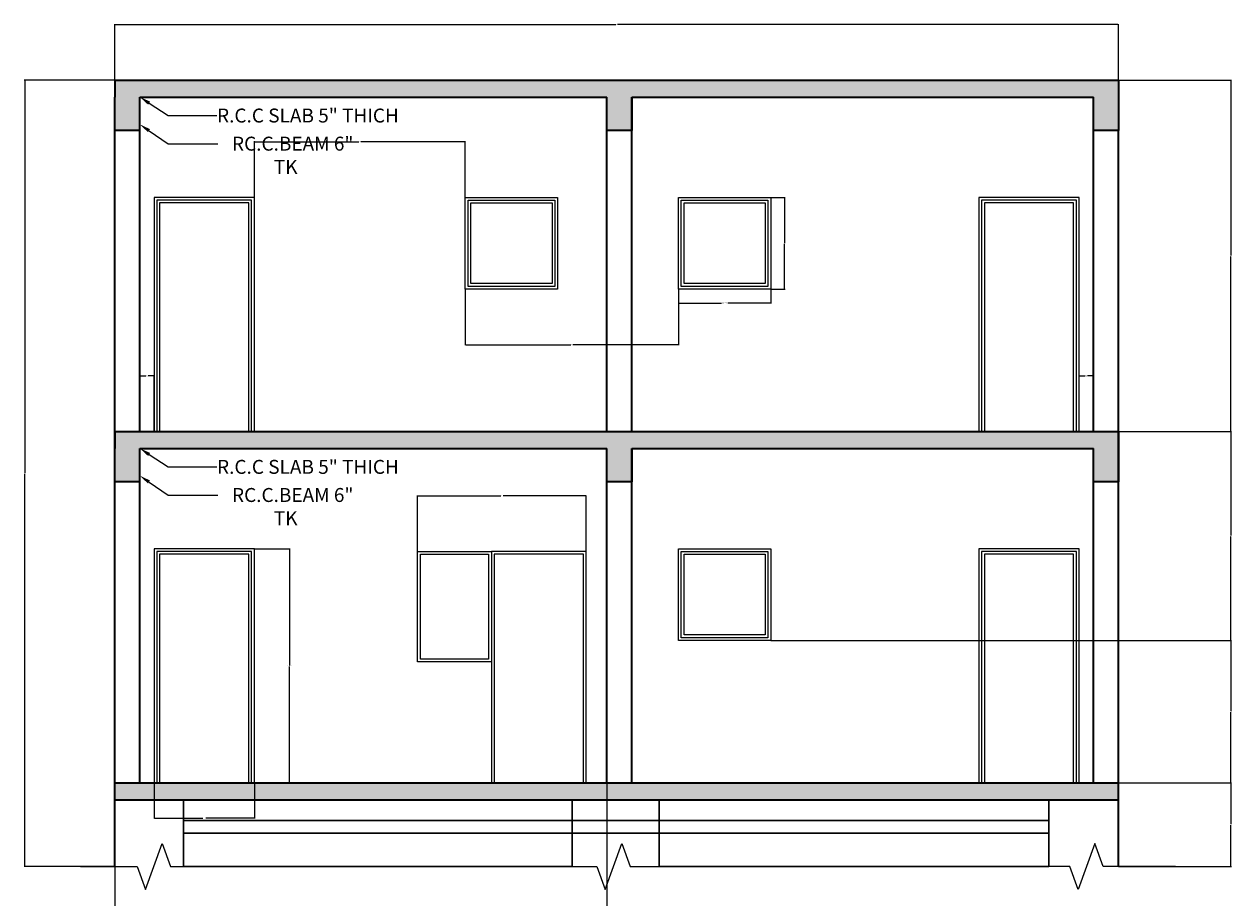
# Model space of a CAD drawing. Units: inches. Extents: x -29 to 834, y -635 to 572.
# Tile 4 of 4: x 401 to 834, y 69 to 383. Entities that reach past the tile are written whole.
import ezdxf
from ezdxf import colors
from ezdxf.entities.mleader import LeaderData, LeaderLine
from ezdxf.math import Vec2, Vec3

# ---------------------------------------------------------------- set-up
doc = ezdxf.new("R2010")
doc.units = ezdxf.units.IN
doc.header["$MEASUREMENT"] = 0
for name, color, linetype, lineweight in [('A-ANNO-DIMS', 2, 'Continuous', 18), ('A-ANNO-SYMB', 2, 'Continuous', 18), ('A-ANNO-TEXT', 7, 'Continuous', 18), ('A-DOOR', 3, 'Continuous', 18), ('A-GLAZ', 4, 'Continuous', 18), ('A-SECT', 7, 'Continuous', 35), ('S-FNDN', 7, 'Continuous', 30), ('S-SLAB', 7, 'Continuous', 35), ('S-SLAB-PATT', 252, 'Continuous', 13)]:
    doc.layers.add(name, color=color, linetype=linetype, lineweight=lineweight)
doc.styles.get("Standard").update_dxf_attribs({"font": 'arial.ttf'})
doc.dimstyles.get("Standard").update_dxf_attribs({"dimtxt": 0.18, "dimasz": 0.18, "dimexe": 0.18, "dimexo": 0.0625, "dimgap": 0.09, "dimtad": 0, "dimtih": 1, "dimtoh": 1, "dimdec": 4, "dimzin": 0, "dimdsep": 46, "dimtxsty": 'Standard', "dimcen": 0.09, "dimadec": 0, "dimazin": 0, "dimtfac": 1, "dimtdec": 4, "dimtofl": 0, "dimtmove": 0, "dimatfit": 3, "dimfxl": 1, "dimtolj": 1, "dimtzin": 0, "dimarcsym": 0})

# ---------------------------------------------------------------- blocks, each defined once
blk = doc.blocks.new('DOOR-36X84-SECT')
for points in [[(36, 0), (36, 84), (0, 84), (0, 0)], [(36, 0), (36, 84), (0, 84), (0, 0)], [(35, 0), (35, 83), (1, 83), (1, 0)], [(34, 0), (34, 82), (2, 82), (2, 0)]]:
    blk.add_lwpolyline(points)
blk = doc.blocks.new('WIN-SQUARE-SECT')
for points in [[(0, 32.92), (33.12, 32.92), (33.12, 0), (0, 0)], [(1, 31.92), (32.12, 31.92), (32.12, 1), (1, 1)], [(2, 30.92), (31.12, 30.92), (31.12, 2), (2, 2)]]:
    blk.add_lwpolyline(points, close=True)
blk = doc.blocks.new('*D55')
at = {"layer": 'A-ANNO-DIMS', "color": 0, "lineweight": -2, "transparency": 16777216}
for p, q in [((483.93, 194.54), (496.65, 194.54)), ((496.47, 194.36), (496.47, 152.72)), ((496.47, 110.72), (496.47, 152.36)), ((483.93, 110.54), (496.65, 110.54))]:
    blk.add_line(p, q, dxfattribs=at)
at = {"layer": 'A-ANNO-DIMS', "color": 0, "transparency": 16777216}
for points in [[(496.44, 194.36), (496.5, 194.36), (496.47, 194.54)], [(496.44, 110.72), (496.5, 110.72), (496.47, 110.54)]]:
    blk.add_solid(points, dxfattribs=at)
at = {"layer": 'DEFPOINTS', "color": 0, "transparency": 16777216}
for p in [(483.87, 194.54), (496.47, 194.54), (483.87, 110.54)]:
    blk.add_point(p, dxfattribs=at)
at = {"layer": 'A-ANNO-DIMS', "color": 0, "transparency": 16777216, "insert": (496.47, 152.54), "char_height": 0.18, "attachment_point": 5}
blk.add_mtext('\\A1;DOOR 84 TYP.', dxfattribs=at)
blk = doc.blocks.new('*D56')
at = {"layer": 'A-ANNO-DIMS', "color": 0, "lineweight": -2, "transparency": 16777216}
for p, q in [((447.87, 110.48), (447.87, 97.76)), ((483.87, 110.48), (483.87, 97.76)), ((448.05, 97.94), (465.34, 97.94)), ((483.69, 97.94), (466.39, 97.94))]:
    blk.add_line(p, q, dxfattribs=at)
at = {"layer": 'A-ANNO-DIMS', "color": 0, "transparency": 16777216}
for points in [[(448.05, 97.97), (448.05, 97.91), (447.87, 97.94)], [(483.69, 97.97), (483.69, 97.91), (483.87, 97.94)]]:
    blk.add_solid(points, dxfattribs=at)
at = {"layer": 'DEFPOINTS', "color": 0, "transparency": 16777216}
for p in [(447.87, 110.54), (483.87, 110.54), (483.87, 97.94)]:
    blk.add_point(p, dxfattribs=at)
at = {"layer": 'A-ANNO-DIMS', "color": 0, "transparency": 16777216, "insert": (465.87, 97.94), "char_height": 0.18, "attachment_point": 5}
blk.add_mtext('\\A1;36 TYP.', dxfattribs=at)
blk = doc.blocks.new('*D57')
at = {"layer": 'A-ANNO-DIMS', "color": 0, "lineweight": -2, "transparency": 16777216}
for p, q in [((635.94, 287.56), (635.94, 282.47)), ((669.06, 287.56), (669.06, 282.47)), ((636.12, 282.65), (651.38, 282.65)), ((668.88, 282.65), (653.62, 282.65))]:
    blk.add_line(p, q, dxfattribs=at)
at = {"layer": 'A-ANNO-DIMS', "color": 0, "transparency": 16777216}
for points in [[(636.12, 282.68), (636.12, 282.62), (635.94, 282.65)], [(668.88, 282.68), (668.88, 282.62), (669.06, 282.65)]]:
    blk.add_solid(points, dxfattribs=at)
at = {"layer": 'DEFPOINTS', "color": 0, "transparency": 16777216}
for p in [(635.94, 287.62), (669.06, 287.62), (669.06, 282.65)]:
    blk.add_point(p, dxfattribs=at)
at = {"layer": 'A-ANNO-DIMS', "color": 0, "transparency": 16777216, "insert": (652.5, 282.65), "char_height": 0.18, "attachment_point": 5}
blk.add_mtext('\\A1;WINDOW 33 TYP.', dxfattribs=at)
blk = doc.blocks.new('*D58')
at = {"layer": 'A-ANNO-DIMS', "color": 0, "lineweight": -2, "transparency": 16777216}
for p, q in [((669.12, 320.54), (674.21, 320.54)), ((674.03, 320.36), (674.03, 304.26)), ((674.03, 287.8), (674.03, 303.9)), ((669.12, 287.62), (674.21, 287.62))]:
    blk.add_line(p, q, dxfattribs=at)
at = {"layer": 'A-ANNO-DIMS', "color": 0, "transparency": 16777216}
for points in [[(674, 320.36), (674.06, 320.36), (674.03, 320.54)], [(674, 287.8), (674.06, 287.8), (674.03, 287.62)]]:
    blk.add_solid(points, dxfattribs=at)
at = {"layer": 'DEFPOINTS', "color": 0, "transparency": 16777216}
for p in [(669.06, 320.54), (674.03, 320.54), (669.06, 287.62)]:
    blk.add_point(p, dxfattribs=at)
at = {"layer": 'A-ANNO-DIMS', "color": 0, "transparency": 16777216, "insert": (674.03, 304.08), "char_height": 0.18, "attachment_point": 5}
blk.add_mtext('\\A1;33 TYP.', dxfattribs=at)
blk = doc.blocks.new('*D95')
at = {"layer": 'A-ANNO-DIMS', "color": 0, "lineweight": -2, "transparency": 16777216}
for p, q in [((433.76, 362.6), (433.76, 382.67)), ((433.94, 382.49), (613.47, 382.49)), ((793.58, 382.49), (614.05, 382.49)), ((793.76, 362.6), (793.76, 382.67))]:
    blk.add_line(p, q, dxfattribs=at)
at = {"layer": 'A-ANNO-DIMS', "color": 0, "transparency": 16777216}
for points in [[(433.94, 382.52), (433.94, 382.46), (433.76, 382.49)], [(793.58, 382.52), (793.58, 382.46), (793.76, 382.49)]]:
    blk.add_solid(points, dxfattribs=at)
at = {"layer": 'DEFPOINTS', "color": 0, "transparency": 16777216}
for p in [(793.76, 382.49), (433.76, 362.54), (793.76, 362.54)]:
    blk.add_point(p, dxfattribs=at)
at = {"layer": 'A-ANNO-DIMS', "color": 0, "transparency": 16777216, "insert": (613.76, 382.49), "char_height": 0.18, "attachment_point": 5}
blk.add_mtext('\\A1;360', dxfattribs=at)
blk = doc.blocks.new('*D96')
at = {"layer": 'A-ANNO-DIMS', "color": 0, "lineweight": -2, "transparency": 16777216}
for p, q in [((433.7, 362.54), (401.3, 362.54)), ((401.48, 362.36), (401.48, 221.72)), ((401.48, 80.72), (401.48, 221.36)), ((433.7, 80.54), (401.3, 80.54))]:
    blk.add_line(p, q, dxfattribs=at)
at = {"layer": 'A-ANNO-DIMS', "color": 0, "transparency": 16777216}
for points in [[(401.45, 362.36), (401.51, 362.36), (401.48, 362.54)], [(401.45, 80.72), (401.51, 80.72), (401.48, 80.54)]]:
    blk.add_solid(points, dxfattribs=at)
at = {"layer": 'DEFPOINTS', "color": 0, "transparency": 16777216}
for p in [(401.48, 362.54), (433.76, 362.54), (433.76, 80.54)]:
    blk.add_point(p, dxfattribs=at)
at = {"layer": 'A-ANNO-DIMS', "color": 0, "transparency": 16777216, "insert": (401.48, 221.54), "char_height": 0.18, "attachment_point": 5}
blk.add_mtext('\\A1;282', dxfattribs=at)
blk = doc.blocks.new('*D97')
at = {"layer": 'A-ANNO-DIMS', "color": 0, "lineweight": -2, "transparency": 16777216}
for p, q in [((793.82, 110.54), (834.3, 110.54)), ((834.12, 110.36), (834.12, 95.72)), ((834.12, 80.72), (834.12, 95.36)), ((793.82, 80.54), (834.3, 80.54))]:
    blk.add_line(p, q, dxfattribs=at)
at = {"layer": 'A-ANNO-DIMS', "color": 0, "transparency": 16777216}
for points in [[(834.09, 110.36), (834.15, 110.36), (834.12, 110.54)], [(834.09, 80.72), (834.15, 80.72), (834.12, 80.54)]]:
    blk.add_solid(points, dxfattribs=at)
at = {"layer": 'DEFPOINTS', "color": 0, "transparency": 16777216}
for p in [(793.76, 110.54), (834.12, 110.54), (793.76, 80.54)]:
    blk.add_point(p, dxfattribs=at)
at = {"layer": 'A-ANNO-DIMS', "color": 0, "transparency": 16777216, "insert": (834.12, 95.54), "char_height": 0.18, "attachment_point": 5}
blk.add_mtext('\\A1;30', dxfattribs=at)
blk = doc.blocks.new('*D98')
at = {"layer": 'A-ANNO-DIMS', "color": 0, "lineweight": -2, "transparency": 16777216}
for p, q in [((669.12, 161.62), (834.3, 161.62)), ((834.12, 161.44), (834.12, 136.26)), ((834.12, 110.72), (834.12, 135.9)), ((793.82, 110.54), (834.3, 110.54))]:
    blk.add_line(p, q, dxfattribs=at)
at = {"layer": 'A-ANNO-DIMS', "color": 0, "transparency": 16777216}
for points in [[(834.09, 161.44), (834.15, 161.44), (834.12, 161.62)], [(834.09, 110.72), (834.15, 110.72), (834.12, 110.54)]]:
    blk.add_solid(points, dxfattribs=at)
at = {"layer": 'DEFPOINTS', "color": 0, "transparency": 16777216}
for p in [(669.06, 161.62), (834.12, 161.62), (793.76, 110.54)]:
    blk.add_point(p, dxfattribs=at)
at = {"layer": 'A-ANNO-DIMS', "color": 0, "transparency": 16777216, "insert": (834.12, 136.08), "char_height": 0.18, "attachment_point": 5}
blk.add_mtext('\\A1;51.08', dxfattribs=at)
blk = doc.blocks.new('*D99')
at = {"layer": 'A-ANNO-DIMS', "color": 0, "lineweight": -2, "transparency": 16777216}
for p, q in [((793.82, 236.54), (834.3, 236.54)), ((834.12, 236.36), (834.12, 199.26)), ((834.12, 161.8), (834.12, 198.9)), ((669.12, 161.62), (834.3, 161.62))]:
    blk.add_line(p, q, dxfattribs=at)
at = {"layer": 'A-ANNO-DIMS', "color": 0, "transparency": 16777216}
for points in [[(834.09, 236.36), (834.15, 236.36), (834.12, 236.54)], [(834.09, 161.8), (834.15, 161.8), (834.12, 161.62)]]:
    blk.add_solid(points, dxfattribs=at)
at = {"layer": 'DEFPOINTS', "color": 0, "transparency": 16777216}
for p in [(793.76, 236.54), (834.12, 236.54), (669.06, 161.62)]:
    blk.add_point(p, dxfattribs=at)
at = {"layer": 'A-ANNO-DIMS', "color": 0, "transparency": 16777216, "insert": (834.12, 199.08), "char_height": 0.18, "attachment_point": 5}
blk.add_mtext('\\A1;74.92', dxfattribs=at)
blk = doc.blocks.new('*D100')
at = {"layer": 'A-ANNO-DIMS', "color": 0, "lineweight": -2, "transparency": 16777216}
for p, q in [((793.82, 362.54), (834.3, 362.54)), ((834.12, 362.36), (834.12, 299.72)), ((834.12, 236.72), (834.12, 299.36)), ((793.82, 236.54), (834.3, 236.54))]:
    blk.add_line(p, q, dxfattribs=at)
at = {"layer": 'A-ANNO-DIMS', "color": 0, "transparency": 16777216}
for points in [[(834.09, 362.36), (834.15, 362.36), (834.12, 362.54)], [(834.09, 236.72), (834.15, 236.72), (834.12, 236.54)]]:
    blk.add_solid(points, dxfattribs=at)
at = {"layer": 'DEFPOINTS', "color": 0, "transparency": 16777216}
for p in [(793.76, 362.54), (834.12, 362.54), (793.76, 236.54)]:
    blk.add_point(p, dxfattribs=at)
at = {"layer": 'A-ANNO-DIMS', "color": 0, "transparency": 16777216, "insert": (834.12, 299.54), "char_height": 0.18, "attachment_point": 5}
blk.add_mtext('\\A1;126', dxfattribs=at)
blk = doc.blocks.new('*D101')
at = {"layer": 'A-ANNO-DIMS', "color": 0, "lineweight": -2, "transparency": 16777216}
for p, q in [((433.76, 110.48), (433.76, 52.17)), ((610.21, 110.48), (610.21, 52.17)), ((433.94, 52.35), (521.53, 52.35)), ((610.03, 52.35), (522.44, 52.35))]:
    blk.add_line(p, q, dxfattribs=at)
at = {"layer": 'A-ANNO-DIMS', "color": 0, "transparency": 16777216}
for points in [[(433.94, 52.38), (433.94, 52.32), (433.76, 52.35)], [(610.03, 52.38), (610.03, 52.32), (610.21, 52.35)]]:
    blk.add_solid(points, dxfattribs=at)
at = {"layer": 'DEFPOINTS', "color": 0, "transparency": 16777216}
for p in [(433.76, 110.54), (610.21, 110.54), (610.21, 52.35)]:
    blk.add_point(p, dxfattribs=at)
at = {"layer": 'A-ANNO-DIMS', "color": 0, "transparency": 16777216, "insert": (521.98, 52.35), "char_height": 0.18, "attachment_point": 5}
blk.add_mtext('\\A1;176.45', dxfattribs=at)
blk = doc.blocks.new('*D102')
at = {"layer": 'A-ANNO-DIMS', "color": 0, "lineweight": -2, "transparency": 16777216}
for p, q in [((442.76, 236.6), (442.76, 256.67)), ((442.94, 256.49), (444.92, 256.49)), ((447.69, 256.49), (445.71, 256.49)), ((447.87, 236.6), (447.87, 256.67))]:
    blk.add_line(p, q, dxfattribs=at)
at = {"layer": 'A-ANNO-DIMS', "color": 0, "transparency": 16777216}
for points in [[(442.94, 256.52), (442.94, 256.46), (442.76, 256.49)], [(447.69, 256.52), (447.69, 256.46), (447.87, 256.49)]]:
    blk.add_solid(points, dxfattribs=at)
at = {"layer": 'DEFPOINTS', "color": 0, "transparency": 16777216}
for p in [(447.87, 256.49), (442.76, 236.54), (447.87, 236.54)]:
    blk.add_point(p, dxfattribs=at)
at = {"layer": 'A-ANNO-DIMS', "color": 0, "transparency": 16777216, "insert": (445.31, 256.49), "char_height": 0.18, "attachment_point": 5}
blk.add_mtext('\\A1;5.106', dxfattribs=at)
blk = doc.blocks.new('*D103')
at = {"layer": 'A-ANNO-DIMS', "color": 0, "lineweight": -2, "transparency": 16777216}
for p, q in [((779.65, 236.6), (779.65, 256.67)), ((779.83, 256.49), (781.81, 256.49)), ((784.58, 256.49), (782.6, 256.49)), ((784.76, 236.6), (784.76, 256.67))]:
    blk.add_line(p, q, dxfattribs=at)
at = {"layer": 'A-ANNO-DIMS', "color": 0, "transparency": 16777216}
for points in [[(779.83, 256.52), (779.83, 256.46), (779.65, 256.49)], [(784.58, 256.52), (784.58, 256.46), (784.76, 256.49)]]:
    blk.add_solid(points, dxfattribs=at)
at = {"layer": 'DEFPOINTS', "color": 0, "transparency": 16777216}
for p in [(784.76, 256.49), (779.65, 236.54), (784.76, 236.54)]:
    blk.add_point(p, dxfattribs=at)
at = {"layer": 'A-ANNO-DIMS', "color": 0, "transparency": 16777216, "insert": (782.21, 256.49), "char_height": 0.18, "attachment_point": 5}
blk.add_mtext('\\A1;5.106', dxfattribs=at)
blk = doc.blocks.new('*D104')
at = {"layer": 'A-ANNO-DIMS', "color": 0, "lineweight": -2, "transparency": 16777216}
for p, q in [((559.48, 287.56), (559.48, 267.49)), ((635.94, 287.56), (635.94, 267.49)), ((559.66, 267.67), (597.32, 267.67)), ((635.76, 267.67), (598.1, 267.67))]:
    blk.add_line(p, q, dxfattribs=at)
at = {"layer": 'A-ANNO-DIMS', "color": 0, "transparency": 16777216}
for points in [[(559.66, 267.7), (559.66, 267.64), (559.48, 267.67)], [(635.76, 267.7), (635.76, 267.64), (635.94, 267.67)]]:
    blk.add_solid(points, dxfattribs=at)
at = {"layer": 'DEFPOINTS', "color": 0, "transparency": 16777216}
for p in [(559.48, 287.62), (635.94, 287.62), (559.48, 267.67)]:
    blk.add_point(p, dxfattribs=at)
at = {"layer": 'A-ANNO-DIMS', "color": 0, "transparency": 16777216, "insert": (597.71, 267.67), "char_height": 0.18, "attachment_point": 5}
blk.add_mtext('\\A1;76.45', dxfattribs=at)
blk = doc.blocks.new('*D105')
at = {"layer": 'A-ANNO-DIMS', "color": 0, "lineweight": -2, "transparency": 16777216}
for p, q in [((483.87, 320.6), (483.87, 340.67)), ((484.05, 340.49), (521.28, 340.49)), ((559.3, 340.49), (522.07, 340.49)), ((559.48, 320.6), (559.48, 340.67))]:
    blk.add_line(p, q, dxfattribs=at)
at = {"layer": 'A-ANNO-DIMS', "color": 0, "transparency": 16777216}
for points in [[(484.05, 340.52), (484.05, 340.46), (483.87, 340.49)], [(559.3, 340.52), (559.3, 340.46), (559.48, 340.49)]]:
    blk.add_solid(points, dxfattribs=at)
at = {"layer": 'DEFPOINTS', "color": 0, "transparency": 16777216}
for p in [(559.48, 340.49), (483.87, 320.54), (559.48, 320.54)]:
    blk.add_point(p, dxfattribs=at)
at = {"layer": 'A-ANNO-DIMS', "color": 0, "transparency": 16777216, "insert": (521.67, 340.49), "char_height": 0.18, "attachment_point": 5}
blk.add_mtext('\\A1;75.62', dxfattribs=at)
blk = doc.blocks.new('*D106')
at = {"layer": 'A-ANNO-DIMS', "color": 0, "lineweight": -2, "transparency": 16777216}
for p, q in [((542.38, 193.6), (542.38, 213.67)), ((542.56, 213.49), (572.23, 213.49)), ((602.69, 213.49), (573.02, 213.49)), ((602.87, 193.6), (602.87, 213.67))]:
    blk.add_line(p, q, dxfattribs=at)
at = {"layer": 'A-ANNO-DIMS', "color": 0, "transparency": 16777216}
for points in [[(542.56, 213.52), (542.56, 213.46), (542.38, 213.49)], [(602.69, 213.52), (602.69, 213.46), (602.87, 213.49)]]:
    blk.add_solid(points, dxfattribs=at)
at = {"layer": 'DEFPOINTS', "color": 0, "transparency": 16777216}
for p in [(602.87, 213.49), (542.38, 193.54), (602.87, 193.54)]:
    blk.add_point(p, dxfattribs=at)
at = {"layer": 'A-ANNO-DIMS', "color": 0, "transparency": 16777216, "insert": (572.62, 213.49), "char_height": 0.18, "attachment_point": 5}
blk.add_mtext('\\A1;60.49', dxfattribs=at)

msp = doc.modelspace()

# ---------------------------------------------------------------- hatches: boundary and pattern name
at = {"layer": 'S-SLAB-PATT'}
h = msp.add_hatch(color=256, dxfattribs=at)
h.dxf.hatch_style = 1
h.paths.add_polyline_path([(619.2079, 356.5416), (784.7594, 356.5416), (784.7594, 344.5416), (793.7594, 344.5416), (793.7594, 362.5416), (433.7594, 362.5416), (433.7594, 356.5416), (433.7594, 344.5416), (442.7594, 344.5416), (442.7594, 356.5416), (610.2079, 356.5416), (610.2079, 344.5416), (619.2079, 344.5416)])
h = msp.add_hatch(color=256, dxfattribs=at)
h.dxf.hatch_style = 1
h.paths.add_polyline_path([(619.2079, 230.5416), (784.7594, 230.5416), (784.7594, 218.5416), (793.7594, 218.5416), (793.7594, 236.5416), (433.7594, 236.5416), (433.7594, 230.5416), (433.7594, 218.5416), (442.7594, 218.5416), (442.7594, 230.5416), (610.2079, 230.5416), (610.2079, 218.5416), (619.2079, 218.5416)])
h = msp.add_hatch(color=256, dxfattribs=at)
h.dxf.hatch_style = 1
h.paths.add_polyline_path([(793.7594, 110.5416), (433.7594, 110.5416), (433.7594, 104.5416), (793.7594, 104.5416)])

# ---------------------------------------------------------------- linework, layer by layer
at = {"layer": 'A-ANNO-SYMB'}
for points in [[(421.4287, 80.5416), (441.8027, 80.5416), (444.8027, 72.2992), (450.8027, 88.784), (453.8027, 80.5416), (467.7819, 80.5416)], [(583.3909, 80.5416), (606.648, 80.5416), (609.648, 72.2992), (615.648, 88.784), (618.648, 80.5416), (641.9051, 80.5416)], [(814.1675, 80.5416), (788.3059, 80.5416), (785.3059, 88.784), (779.3059, 72.2992), (776.3059, 80.5416), (758.866, 80.5416)]]:
    msp.add_lwpolyline(points, dxfattribs=at)
at = {"layer": 'A-DOOR'}
for points in [[(602.868, 110.5416), (602.868, 193.5416), (568.868, 193.5416), (568.868, 110.5416)], [(601.868, 110.5416), (601.868, 192.5416), (569.868, 192.5416), (569.868, 110.5416)]]:
    msp.add_lwpolyline(points, dxfattribs=at)
at = {"layer": 'A-GLAZ'}
for points in [[(542.3815, 193.5416), (568.868, 193.5416), (568.868, 153.9833), (542.3815, 153.9833)], [(543.3815, 192.5416), (567.868, 192.5416), (567.868, 154.9833), (543.3815, 154.9833)]]:
    msp.add_lwpolyline(points, close=True, dxfattribs=at)
at = {"layer": 'A-SECT'}
for p, q in [((433.7594, 206.5416), (433.7594, 356.5416)), ((442.7594, 236.5416), (442.7594, 356.5416)), ((610.2079, 236.5416), (610.2079, 356.5416)), ((619.2079, 236.5416), (619.2079, 356.5416)), ((784.7594, 236.5416), (784.7594, 356.5416)), ((793.7594, 206.5416), (793.7594, 344.5416)), ((433.7594, 80.5416), (433.7594, 230.5416)), ((442.7594, 110.5416), (442.7594, 230.5416)), ((610.2079, 110.5416), (610.2079, 230.5416)), ((619.2079, 110.5416), (619.2079, 230.5416)), ((784.7594, 110.5416), (784.7594, 230.5416)), ((793.7594, 80.5416), (793.7594, 218.5416))]:
    msp.add_line(p, q, dxfattribs=at)
at = {"layer": 'S-FNDN'}
for p, q in [((458.4302, 104.5416), (458.4302, 80.5416)), ((597.8658, 104.5416), (597.8658, 80.5416)), ((629.0546, 104.5416), (629.0546, 80.5416)), ((768.7594, 80.5416), (768.7594, 104.5416)), ((458.4302, 97.0887), (768.7594, 97.0887)), ((458.4302, 92.5416), (768.7594, 92.5416)), ((458.4302, 80.5416), (597.8658, 80.5416)), ((629.0546, 80.5416), (768.7594, 80.5416))]:
    msp.add_line(p, q, dxfattribs=at)
at = {"layer": 'S-SLAB'}
for p, q in [((433.7594, 362.5416), (793.7594, 362.5416)), ((433.7594, 362.5416), (433.7594, 356.5416)), ((793.7594, 362.5416), (793.7594, 344.5416)), ((442.7594, 356.5416), (610.2079, 356.5416)), ((619.2079, 356.5416), (784.7594, 356.5416)), ((619.2079, 356.5416), (619.2079, 344.5416)), ((442.7594, 344.5416), (433.7594, 344.5416)), ((619.2079, 344.5416), (610.2079, 344.5416)), ((793.7594, 344.5416), (784.7594, 344.5416)), ((433.7594, 236.5416), (793.7594, 236.5416)), ((433.7594, 236.5416), (433.7594, 230.5416)), ((793.7594, 236.5416), (793.7594, 218.5416)), ((442.7594, 230.5416), (610.2079, 230.5416)), ((619.2079, 230.5416), (619.2079, 218.5416)), ((619.2079, 230.5416), (784.7594, 230.5416)), ((442.7594, 218.5416), (433.7594, 218.5416)), ((619.2079, 218.5416), (610.2079, 218.5416)), ((793.7594, 218.5416), (784.7594, 218.5416)), ((433.7594, 110.5416), (793.7594, 110.5416)), ((433.7594, 104.5416), (793.7594, 104.5416))]:
    msp.add_line(p, q, dxfattribs=at)

# ---------------------------------------------------------------- block references
at = {"layer": 'A-DOOR'}
for p in [(447.8652, 236.5416), (743.6537, 236.5416), (447.8652, 110.5416), (743.6537, 110.5416)]:
    msp.add_blockref('DOOR-36X84-SECT', p, dxfattribs=at)
at = {"layer": 'A-GLAZ'}
for p in [(559.4833, 287.6203), (635.9367, 287.6203), (635.9367, 161.6203)]:
    msp.add_blockref('WIN-SQUARE-SECT', p, dxfattribs=at)

# ---------------------------------------------------------------- dimensions: what is measured, and where the dimension line sits
at = {"layer": 'A-ANNO-DIMS'}
for base, p1, p2, override, picture, middle in [((793.7594, 382.4916), (433.7594, 362.5416), (793.7594, 362.5416), {"dimdec": 0, "dimlfac": 1, "dimrnd": 0, "dimzin": 0, "dimdsep": 46, "dimlunit": 2}, '*D95', (613.7594, 382.4916)), ((559.4833, 340.4916), (483.8652, 320.5416), (559.4833, 320.5416), {"dimdec": 2, "dimlfac": 1, "dimrnd": 0, "dimzin": 0, "dimdsep": 46, "dimlunit": 2}, '*D105', (521.6742, 340.4916)), ((784.7594, 256.4916), (779.6537, 236.5416), (784.7594, 236.5416), {"dimdec": 3, "dimlfac": 1, "dimrnd": 0, "dimzin": 0, "dimdsep": 46, "dimlunit": 2}, '*D103', (782.2066, 256.4916)), ((602.868, 213.4916), (542.3815, 193.5416), (602.868, 193.5416), {"dimdec": 2, "dimlfac": 1, "dimrnd": 0, "dimzin": 0, "dimdsep": 46, "dimlunit": 2}, '*D106', (572.6248, 213.4916)), ((610.2079, 52.3492), (433.7594, 110.5416), (610.2079, 110.5416), {"dimdec": 2, "dimlfac": 1, "dimrnd": 0, "dimzin": 0, "dimdsep": 46, "dimlunit": 2}, '*D101', (521.9837, 52.3492))]:
    dim = msp.add_linear_dim(base=base, p1=p1, p2=p2, dimstyle='Standard', override=override, dxfattribs=at)
    dim.commit()
    dim.dimension.update_dxf_attribs({"geometry": picture, "text_midpoint": middle})
for base, p1, p2, angle, override, picture, middle in [((401.4787, 362.5416), (433.7594, 80.5416), (433.7594, 362.5416), 90, {"dimdec": 0, "dimlfac": 1, "dimrnd": 0, "dimzin": 0, "dimdsep": 46, "dimlunit": 2}, '*D96', (401.4787, 221.5416)), ((834.1175, 362.5416), (793.7594, 236.5416), (793.7594, 362.5416), 90, {"dimdec": 0, "dimlfac": 1, "dimrnd": 0, "dimzin": 0, "dimdsep": 46, "dimlunit": 2}, '*D100', (834.1175, 299.5416)), ((559.4833, 267.6703), (635.9367, 287.6203), (559.4833, 287.6203), 180, {"dimdec": 2, "dimlfac": 1, "dimrnd": 0, "dimzin": 0, "dimdsep": 46, "dimlunit": 2}, '*D104', (597.71, 267.6703)), ((447.8652, 256.4916), (442.7594, 236.5416), (447.8652, 236.5416), 0, {"dimdec": 3, "dimlfac": 1, "dimrnd": 0, "dimzin": 0, "dimdsep": 46, "dimlunit": 2}, '*D102', (445.3123, 256.4916)), ((834.1175, 236.5416), (669.0587, 161.6203), (793.7594, 236.5416), 90, {"dimdec": 2, "dimlfac": 1, "dimrnd": 0, "dimzin": 0, "dimdsep": 46, "dimlunit": 2}, '*D99', (834.1175, 199.081)), ((834.1175, 161.6203), (793.7594, 110.5416), (669.0587, 161.6203), 90, {"dimdec": 2, "dimlfac": 1, "dimrnd": 0, "dimzin": 0, "dimdsep": 46, "dimlunit": 2}, '*D98', (834.1175, 136.081)), ((834.1175, 110.5416), (793.7594, 80.5416), (793.7594, 110.5416), 90, {"dimdec": 0, "dimlfac": 1, "dimrnd": 0, "dimzin": 0, "dimdsep": 46, "dimlunit": 2}, '*D97', (834.1175, 95.5416))]:
    dim = msp.add_linear_dim(base=base, p1=p1, p2=p2, angle=angle, dimstyle='Standard', override=override, dxfattribs=at)
    dim.commit()
    dim.dimension.update_dxf_attribs({"geometry": picture, "text_midpoint": middle})
for base, p1, p2, text, picture, middle in [((674.027, 320.5416), (669.0587, 287.6203), (669.0587, 320.5416), '<> TYP.', '*D58', (674.027, 304.081)), ((496.4652, 194.5416), (483.8652, 110.5416), (483.8652, 194.5416), 'DOOR <> TYP.', '*D55', (496.4652, 152.5416))]:
    dim = msp.add_linear_dim(base=base, p1=p1, p2=p2, angle=90, text=text, dimstyle='Standard', override={"dimdec": 0, "dimlfac": 1, "dimrnd": 0, "dimzin": 0, "dimdsep": 46, "dimlunit": 2}, dxfattribs=at)
    dim.commit()
    dim.dimension.update_dxf_attribs({"geometry": picture, "text_midpoint": middle})
for base, p1, p2, text, picture, middle in [((669.0587, 282.652), (635.9367, 287.6203), (669.0587, 287.6203), 'WINDOW <> TYP.', '*D57', (652.4977, 282.652)), ((483.8652, 97.9416), (447.8652, 110.5416), (483.8652, 110.5416), '<> TYP.', '*D56', (465.8652, 97.9416))]:
    dim = msp.add_linear_dim(base=base, p1=p1, p2=p2, text=text, dimstyle='Standard', override={"dimdec": 0, "dimlfac": 1, "dimrnd": 0, "dimzin": 0, "dimdsep": 46, "dimlunit": 2}, dxfattribs=at)
    dim.commit()
    dim.dimension.update_dxf_attribs({"geometry": picture, "text_midpoint": middle})

# ---------------------------------------------------------------- leaders
at = {"layer": 'A-ANNO-TEXT'}
ml = msp.add_multileader_mtext('Standard', dxfattribs=at)
ml.set_content('R.C.C SLAB 5" THICH', color=256)
ml.set_leader_properties()
ml.build(insert=Vec2(0, 0))
ml.multileader.update_dxf_attribs({"dogleg_length": 0.36})
ctx = ml.context
ctx.base_point, ctx.char_height, ctx.landing_gap_size, ctx.plane_origin = Vec3(470.3678, 349.8613), 5, 0.09, Vec3(442.7594, 356.5416)
notes = []
notes.append((ctx, [(0, (1, 1, 0), (470.0078, 349.8613), (1, 0), 0.36, [(0, [(442.7594, 356.5416), (452.8812, 349.8613)], 0, [])])]))
ctx.mtext.insert, ctx.mtext.flow_direction = Vec3(470.4578, 352.4039), 5
ml = msp.add_multileader_mtext('Standard', dxfattribs=at)
ml.set_content('\\pxi-3,l4,t4;RC.C.BEAM 6" TK', color=256)
ml.set_leader_properties()
ml.build(insert=Vec2(0, 0))
ml.multileader.update_dxf_attribs({"dogleg_length": 0.36})
ctx = ml.context
ctx.base_point, ctx.char_height, ctx.landing_gap_size, ctx.plane_origin = Vec3(470.7278, 339.7718), 5, 0.09, Vec3(442.7594, 346.7341)
notes.append((ctx, [(0, (1, 1, 0), (470.3678, 339.7718), (1, 0), 0.36, [(0, [(442.7594, 346.7341), (452.8812, 339.7718)], 0, [])])]))
ctx.mtext.insert, ctx.mtext.flow_direction = Vec3(470.8178, 342.3144), 5
ml = msp.add_multileader_mtext('Standard', dxfattribs=at)
ml.set_content('R.C.C SLAB 5" THICH', color=256)
ml.set_leader_properties()
ml.build(insert=Vec2(0, 0))
ml.multileader.update_dxf_attribs({"dogleg_length": 0.36})
ctx = ml.context
ctx.base_point, ctx.char_height, ctx.landing_gap_size, ctx.plane_origin = Vec3(470.3678, 223.8613), 5, 0.09, Vec3(442.7594, 230.5416)
notes.append((ctx, [(0, (1, 1, 0), (470.0078, 223.8613), (1, 0), 0.36, [(0, [(442.7594, 230.5416), (452.8812, 223.8613)], 0, [])])]))
ctx.mtext.insert, ctx.mtext.flow_direction = Vec3(470.4578, 226.4039), 5
ml = msp.add_multileader_mtext('Standard', dxfattribs=at)
ml.set_content('\\pxi-3,l4,t4;RC.C.BEAM 6" TK', color=256)
ml.set_leader_properties()
ml.build(insert=Vec2(0, 0))
ml.multileader.update_dxf_attribs({"dogleg_length": 0.36})
ctx = ml.context
ctx.base_point, ctx.char_height, ctx.landing_gap_size, ctx.plane_origin = Vec3(470.7278, 213.7718), 5, 0.09, Vec3(442.7594, 220.7341)
notes.append((ctx, [(0, (1, 1, 0), (470.3678, 213.7718), (1, 0), 0.36, [(0, [(442.7594, 220.7341), (452.8812, 213.7718)], 0, [])])]))
ctx.mtext.insert, ctx.mtext.flow_direction = Vec3(470.8178, 216.3144), 5
for ctx, leaders in notes:
    for number, flags, end, landing, length, lines in leaders:
        leader = LeaderData()
        leader.index, (leader.has_last_leader_line, leader.has_dogleg_vector, leader.attachment_direction) = number, flags
        leader.last_leader_point, leader.dogleg_vector, leader.dogleg_length = Vec3(end), Vec3(landing), length
        for number, points, colour, breaks in lines:
            line = LeaderLine()
            line.index, line.vertices, line.color, line.breaks = number, Vec3.list(points), colors.encode_raw_color(colour), breaks
            leader.lines.append(line)
        ctx.leaders.append(leader)

doc.saveas('drawing.dxf')
